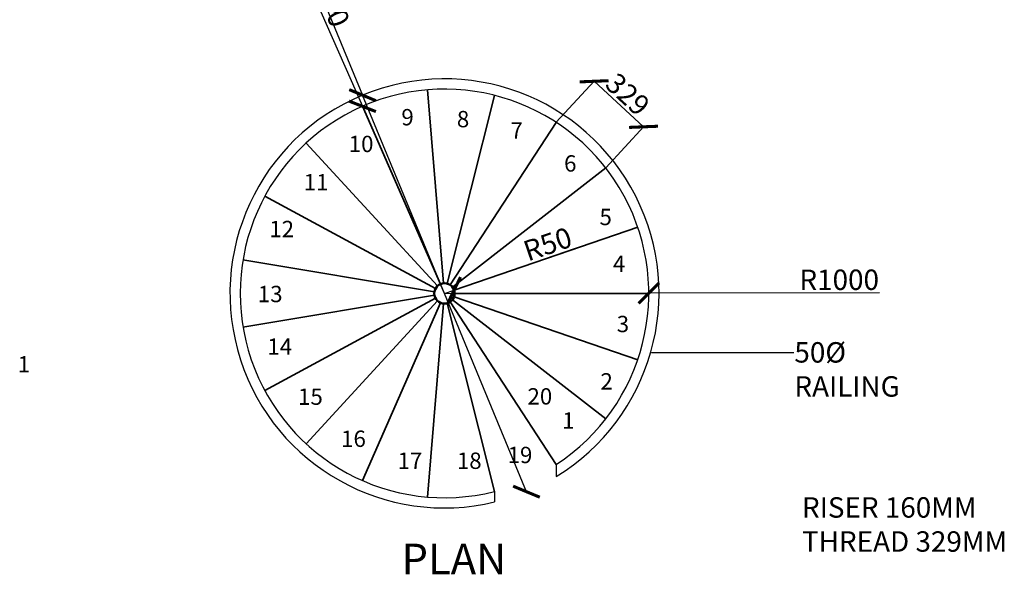
# Model space of a CAD drawing. Units: millimetres. Extents: x 210 to 5648, y 83 to 7906.
# Tile 1 of 2: x 828 to 5648, y 83 to 2798. Entities that reach past the tile are written whole.
import ezdxf
from ezdxf import colors
from ezdxf.entities.mleader import LeaderData, LeaderLine
from ezdxf.math import Vec2, Vec3

# ---------------------------------------------------------------- set-up
doc = ezdxf.new("R2010")
doc.units = ezdxf.units.MM
for name, color, linetype, lineweight in [('A-ANNO-DIMS', 2, 'Continuous', 18), ('A-ANNO-TEXT', 240, 'Continuous', 18), ('A-COLS', 1, 'Continuous', 50), ('A-FLOR-HRAL', 4, 'Continuous', 25), ('A-FLOR-STRS', 7, 'Continuous', 35)]:
    doc.layers.add(name, color=color, linetype=linetype, lineweight=lineweight)
doc.styles.get("Standard").update_dxf_attribs({"font": 'arial.ttf'})
doc.dimstyles.new('ISO-25', dxfattribs={"dimtxt": 100, "dimasz": 100, "dimexe": 1.25, "dimexo": 0.625, "dimtad": 1, "dimtxsty": 'Standard', "dimblk": 'ARCHTICK', "dimcen": 2.5, "dimclrd": 2, "dimclre": 5, "dimclrt": 1, "dimadec": 0, "dimazin": 0, "dimtfac": 1, "dimtmove": 0, "dimatfit": 3, "dimfxl": 1, "dimarcsym": 0})

# ---------------------------------------------------------------- blocks, each defined once
blk = doc.blocks.new('*U1')
blk.add_line((-475, 0), (475, 0))
blk = doc.blocks.new('*U2')
at = {"layer": 'A-FLOR-STRS', "color": 0, "linetype": 'ByBlock', "lineweight": -2, "transparency": 16777216}
for p, rotation in [((2864, 1980.9), 94.73684210526307), ((3036.3, 1966.7), 75.78947368421042), ((2696.5, 1938.5), 113.6842105263156), ((3194.6, 1897.2), 56.8421052631578), ((2551.8, 1844), 132.6315789473682), ((3321.7, 1780.2), 37.89473684210519), ((2445.7, 1707.6), 151.5789473684208), ((3404, 1628.2), 18.94736842105258), ((2389.6, 1544.1), 170.5263157894734), ((2389.6, 1371.3), 189.473684210526), ((2445.7, 1207.9), 208.4210526315786), ((2551.8, 1071.5), 227.3684210526312), ((2696.5, 976.9), 246.3157894736838), ((2864, 934.5), 265.2631578947364), ((3036.3, 948.8), 284.210526315789), ((3194.6, 1018.2), 303.1578947368416), ((3321.7, 1135.3), 322.1052631578943), ((3404, 1287.3), 341.0526315789469)]:
    blk.add_blockref('*U1', p, dxfattribs=dict(at, rotation=rotation))
blk.add_blockref('*U1', (3432.4, 1457.7), dxfattribs=at)
blk = doc.blocks.new('_ArchTick')
at = {"color": 0, "linetype": 'ByBlock', "const_width": 0.15}
blk.add_lwpolyline([(-0.5, -0.5), (0.5, 0.5)], dxfattribs=at)
blk = doc.blocks.new('*D6')
at = {"layer": 'A-ANNO-DIMS', "color": 0, "lineweight": -2, "transparency": 16777216}
for p, q in [((3454.8, 2295.4), (3640.4, 2497.1)), ((3639.6, 2496.1), (3881.8, 2273.2)), ((3697, 2072.4), (3882.6, 2274.1))]:
    blk.add_line(p, q, dxfattribs=at)
at = {"layer": 'Defpoints', "color": 0, "transparency": 16777216}
for p in [(3454.4, 2294.9), (3881.8, 2273.2), (3696.5, 2071.9)]:
    blk.add_point(p, dxfattribs=at)
at = {"layer": 'A-ANNO-DIMS', "color": 0, "lineweight": -2, "transparency": 16777216, "xscale": 100, "yscale": 100, "zscale": 100}
for p, rotation in [((3639.6, 2496.1), 137.3684210526315), ((3881.8, 2273.2), 317.3684210526316)]:
    blk.add_blockref('_ArchTick', p, dxfattribs=dict(at, rotation=rotation))
at = {"layer": 'A-ANNO-DIMS', "color": 0, "transparency": 16777216, "insert": (3795.7, 2422.7), "char_height": 100, "attachment_point": 5, "rotation": 317.3684}
blk.add_mtext('329', dxfattribs=at)
blk = doc.blocks.new('*D7')
at = {"layer": 'A-ANNO-DIMS', "color": 0, "lineweight": -2, "transparency": 16777216}
for p in [(2907.4, 1457.7), (5037.2, 1460.2)]:
    blk.add_line(p, (3907.4, 1458.9), dxfattribs=at)
at = {"layer": 'Defpoints', "color": 0, "transparency": 16777216}
for p in [(2907.4, 1457.7), (3907.4, 1458.9)]:
    blk.add_point(p, dxfattribs=at)
at = {"layer": 'A-ANNO-DIMS', "color": 0, "lineweight": -2, "transparency": 16777216, "xscale": 100, "yscale": 100, "zscale": 100, "rotation": 180.0661597744912}
blk.add_blockref('_ArchTick', (3907.4, 1458.9), dxfattribs=at)
at = {"layer": 'A-ANNO-DIMS', "color": 0, "transparency": 16777216, "insert": (4839.5, 1511.6), "char_height": 100, "attachment_point": 5, "rotation": 0.0662}
blk.add_mtext('R1000', dxfattribs=at)
blk = doc.blocks.new('*D8')
at = {"layer": 'A-ANNO-DIMS', "color": 0, "lineweight": -2, "transparency": 16777216}
for p in [(3546.6, 1677.2), (2907.4, 1457.7)]:
    blk.add_line(p, (2954.7, 1474), dxfattribs=at)
at = {"layer": 'Defpoints', "color": 0, "transparency": 16777216}
for p in [(2907.4, 1457.7), (2954.7, 1474)]:
    blk.add_point(p, dxfattribs=at)
at = {"layer": 'A-ANNO-DIMS', "color": 0, "lineweight": -2, "transparency": 16777216, "xscale": 100, "yscale": 100, "zscale": 100, "rotation": 198.9473684210503}
blk.add_blockref('_ArchTick', (2954.7, 1474), dxfattribs=at)
at = {"layer": 'A-ANNO-DIMS', "color": 0, "transparency": 16777216, "insert": (3416.4, 1687.1), "char_height": 100, "attachment_point": 5, "rotation": 18.9474}
blk.add_mtext('R50', dxfattribs=at)
blk = doc.blocks.new('*D16')
at = {"layer": 'A-ANNO-DIMS', "color": 2, "lineweight": -2, "transparency": 16777216}
for p in [(2187.7, 3199), (3308.5, 487.3)]:
    blk.add_line(p, (2506.3, 2428.1), dxfattribs=at)
at = {"layer": 'Defpoints', "color": 0, "transparency": 16777216}
for p in [(2506.3, 2428.1), (3308.5, 487.3)]:
    blk.add_point(p, dxfattribs=at)
at = {"layer": 'A-ANNO-DIMS', "color": 2, "lineweight": -2, "transparency": 16777216, "xscale": 100, "yscale": 100, "zscale": 100}
for p, rotation in [((2506.3, 2428.1), 292.4567190753457), ((3308.5, 487.3), 112.4567190753456)]:
    blk.add_blockref('_ArchTick', p, dxfattribs=dict(at, rotation=rotation))
at = {"layer": 'A-ANNO-DIMS', "color": 1, "transparency": 16777216, "insert": (2316, 3031.1), "char_height": 100, "attachment_point": 5, "rotation": 292.4567}
blk.add_mtext('∅2100', dxfattribs=at)
blk = doc.blocks.new('*D17')
at = {"layer": 'A-ANNO-DIMS', "color": 2, "lineweight": -2, "transparency": 16777216}
for p in [(2185.3, 3103.9), (2907.4, 1457.7)]:
    blk.add_line(p, (2505.7, 2373.5), dxfattribs=at)
at = {"layer": 'Defpoints', "color": 0, "transparency": 16777216}
for p in [(2505.7, 2373.5), (2907.4, 1457.7)]:
    blk.add_point(p, dxfattribs=at)
at = {"layer": 'A-ANNO-DIMS', "color": 2, "lineweight": -2, "transparency": 16777216, "xscale": 100, "yscale": 100, "zscale": 100, "rotation": 293.6842151788714}
blk.add_blockref('_ArchTick', (2505.7, 2373.5), dxfattribs=at)
at = {"layer": 'A-ANNO-DIMS', "color": 1, "transparency": 16777216, "insert": (2312, 2943.7), "char_height": 100, "attachment_point": 5, "rotation": 293.6842}
blk.add_mtext('R1000', dxfattribs=at)

msp = doc.modelspace()

# ---------------------------------------------------------------- linework, layer by layer
at = {"layer": 'A-COLS'}
msp.add_circle((2907.403, 1457.726), 50, dxfattribs=at)
at = {"layer": 'A-FLOR-HRAL'}
for p, q in [((3454.351, 620.56), (3454.351, 561.43)), ((3152.888, 488.326), (3152.888, 436.826))]:
    msp.add_line(p, q, dxfattribs=at)
for radius, start, end in [(1050, 301.392843, 283.520644), (1000, 303.157895, 284.210526)]:
    msp.add_arc((2907.403, 1457.726), radius, start, end, dxfattribs=at)

# ---------------------------------------------------------------- block references
at = {"layer": 'A-FLOR-STRS'}
msp.add_blockref('*U2', (0, 0), dxfattribs=at)

# ---------------------------------------------------------------- texts
at = {"layer": 'A-ANNO-TEXT', "attachment_point": 1}
for s, width, insert, char_height in [('9', 220.13349, (2696.319, 2360.374), 80), ('8', 220.13349, (2967.973, 2351.018), 80), ('7', 220.13349, (3230.26, 2294.878), 80), ('10', 220.13349, (2438.716, 2229.382), 80), ('6', 220.13349, (3492.846, 2134.026), 80), ('11', 220.13349, (2218.583, 2042.25), 80), ('5', 220.13349, (3666.143, 1872.041), 80), ('12', 220.13349, (2049.97, 1813.013), 80), ('4', 220.13349, (3731.715, 1642.804), 80), ('13', 220.13349, (1993.765, 1494.888), 80), ('3', 220.13349, (3750.449, 1348.071), 80), ('14', 220.13349, (2040.602, 1237.581), 80), ('1', 220.13349, (818.458, 1150.786), 80), ('2', 220.13349, (3670.826, 1067.373), 80), ('15', 220.13349, (2190.588, 992.329), 80), ('20', 220.13349, (3313.598, 993.908), 80), ('1', 220.13349, (3483.479, 875.562), 80), ('16', 220.13349, (2401.354, 786.484), 80), ('17', 220.13349, (2677.692, 678.883), 80), ('18', 220.13349, (2968.081, 678.883), 80), ('19', 220.13349, (3216.316, 706.953), 80), ('RISER 160MM\\PTHREAD 329MM', 1234.99387, (4657.246, 460.117), 100)]:
    msp.add_mtext_dynamic_manual_height_columns(s, width=width, gutter_width=12.5, heights=[0], dxfattribs=dict(at, insert=insert, char_height=char_height))
at = {"layer": 'A-ANNO-TEXT', "insert": (2697.174, 232.854), "char_height": 150, "width": 1326.11889, "attachment_point": 1}
msp.add_mtext('{\\fArial|b1|i0|c0|p34;PLAN}', dxfattribs=at)

# ---------------------------------------------------------------- dimensions: what is measured, and where the dimension line sits
at = {"layer": 'A-ANNO-DIMS'}
dim = msp.add_diameter_dim_2p(p1=(3308.487, 487.35), p2=(2506.318, 2428.103), dimstyle='ISO-25', override={"dimdec": 0, "dimlfac": 1, "dimrnd": 0, "dimzin": 0, "dimdsep": 46, "dimlunit": 2}, dxfattribs=at)
dim.commit()
dim.dimension.update_dxf_attribs({"geometry": '*D16', "text_midpoint": (2265.667, 3010.329), "dimtype": 163})
for mpoint, override, picture, middle in [((2505.707, 2373.5), {"dimdec": 0, "dimlfac": 1, "dimrnd": 0, "dimzin": 0, "dimdsep": 46, "dimlunit": 2}, '*D17', (2264.69, 2922.964)), ((2954.694, 1473.961), {"dimclrd": 0, "dimclre": 0, "dimclrt": 0}, '*D8', (3433.151, 1638.216)), ((3907.402, 1458.881), {"dimclrd": 0, "dimclre": 0, "dimclrt": 0}, '*D7', (4839.562, 1459.957))]:
    dim = msp.add_radius_dim(center=(2907.403, 1457.726), mpoint=mpoint, dimstyle='ISO-25', override=override, dxfattribs=at)
    dim.commit()
    dim.dimension.update_dxf_attribs({"geometry": picture, "text_midpoint": middle, "dimtype": 164})
dim = msp.add_aligned_dim(p1=(3454.351, 2294.893), p2=(3696.543, 2071.939), distance=273.523, text='329', dimstyle='ISO-25', override={"dimclrd": 0, "dimclre": 0, "dimclrt": 0}, dxfattribs=at)
dim.commit()
dim.dimension.update_dxf_attribs({"geometry": '*D6', "text_midpoint": (3795.726, 2422.703)})

# ---------------------------------------------------------------- leaders
at = {"layer": 'A-ANNO-TEXT'}
ml = msp.add_multileader_mtext('Standard', dxfattribs=at)
ml.set_content('{\\C240;\\c2367469;50%%C RAILIN}G', color=256)
ml.set_leader_properties()
ml.build(insert=Vec2(0, 0))
ctx = ml.context
ctx.base_point, ctx.char_height, ctx.plane_origin = Vec3(4618.009, 1168.299), 100, Vec3(3916.725, 1168.299)
notes = []
notes.append((ctx, [(0, (1, 1, 0), (4610.009, 1168.299), (1, 0), 8, [(0, [(3916.725, 1168.299)], 0, [])])]))
ctx.mtext.insert, ctx.mtext.width, ctx.mtext.flow_direction = Vec3(4620.009, 1219.151), 70.70181, 5
for ctx, leaders in notes:
    for number, flags, end, landing, length, lines in leaders:
        leader = LeaderData()
        leader.index, (leader.has_last_leader_line, leader.has_dogleg_vector, leader.attachment_direction) = number, flags
        leader.last_leader_point, leader.dogleg_vector, leader.dogleg_length = Vec3(end), Vec3(landing), length
        for number, points, colour, breaks in lines:
            line = LeaderLine()
            line.index, line.vertices, line.color, line.breaks = number, Vec3.list(points), colors.encode_raw_color(colour), breaks
            leader.lines.append(line)
        ctx.leaders.append(leader)

doc.saveas('drawing.dxf')
